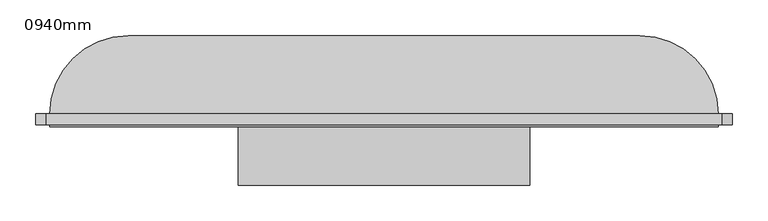
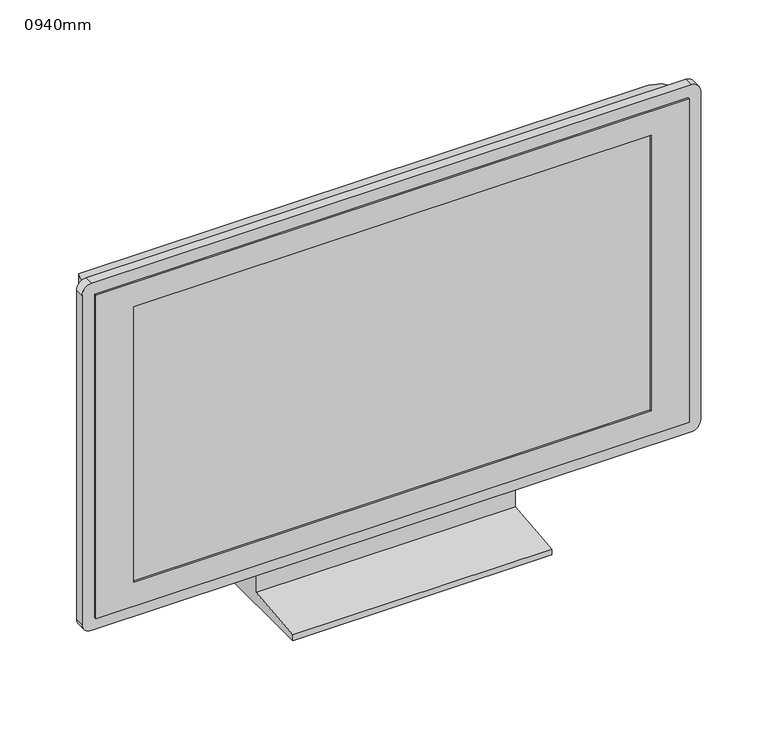
"""IFC4 building model written with IfcOpenShell, lengths in millimetres: furniture geometry, 0940mm."""

from ifc_helpers import new_model, si_unit, point, frame, frame_2d, origin, place, context, project, spatial, polyline, circle_curve, ellipse_curve, trimmed, segment, composite_curve, outline, extrude, faceted_brep, source, transform, mapped, element, save
from ifc_brep_helpers import plane_surface, cylinder_surface, advanced_brep


def furniture_0940mm_4831bac8(model_context):
    return source(origin(), model_context, "Body", "SolidModel", [
        extrude(outline(polyline([(-51.4613764, 80.0), (-1.4613764, 80.0), (48.5386236, 0.0), (-151.4613764, 0.0), (-151.4613764, 10.0), (-51.4613764, 20.0), (-51.4613764, 80.0)])), frame((-208.760248, 0.0, 0.0), z_axis=(1.0, 0.0, 0.0), x_axis=(0.0, 1.0, 0.0)), (0.0, 0.0, 1.0), 409.6314677),
        faceted_brep([(465.6869536, -69.4613764, 620.8776873), (-473.5759818, -69.4613764, 620.8776873), (-473.5759818, -69.4613764, 80.0), (465.6869536, -69.4613764, 80.0), (-413.5759818, -69.4613764, 580.8776873), (405.6869536, -69.4613764, 580.8776873), (405.6869536, -69.4613764, 120.0), (-413.5759818, -69.4613764, 120.0), (465.6869536, -51.4613764, 620.8776873), (465.6869536, -51.4613764, 80.0), (-473.5759818, -51.4613764, 80.0), (-473.5759818, -51.4613764, 620.8776873), (-413.5759818, -66.4613764, 580.8776873), (-413.5759818, -66.4613764, 120.0), (405.6869536, -66.4613764, 120.0), (405.6869536, -66.4613764, 580.8776873)], [[[0, 1, 2, 3], [4, 5, 6, 7]], [[8, 9, 10, 11]], [[1, 0, 8, 11]], [[2, 1, 11, 10]], [[3, 2, 10, 9]], [[0, 3, 9, 8]], [[12, 13, 14, 15]], [[12, 15, 5, 4]], [[15, 14, 6, 5]], [[14, 13, 7, 6]], [[13, 12, 4, 7]]]),
        extrude(outline(composite_curve([segment(polyline([(640.8776873, 470.6869536), (640.8776873, -478.5759818)]), True, "CONTINUOUS"), segment(trimmed(circle_curve(frame_2d((625.8776873, -478.5759818)), 15.0), [point((640.8776873, -478.5759818))], [point((625.8776873, -493.5759818))], False, "CARTESIAN"), True, "CONTINUOUS"), segment(polyline([(625.8776873, -493.5759818), (75.0, -493.5759818)]), True, "CONTINUOUS"), segment(trimmed(circle_curve(frame_2d((75.0, -478.5759818)), 15.0), [point((75.0, -493.5759818))], [point((60.0, -478.5759818))], False, "CARTESIAN"), True, "CONTINUOUS"), segment(polyline([(60.0, -478.5759818), (60.0, 470.6869536)]), True, "CONTINUOUS"), segment(trimmed(circle_curve(frame_2d((75.0, 470.6869536)), 15.0), [point((60.0, 470.6869536))], [point((75.0, 485.6869536))], False, "CARTESIAN"), True, "CONTINUOUS"), segment(polyline([(75.0, 485.6869536), (625.8776873, 485.6869536)]), True, "CONTINUOUS"), segment(trimmed(circle_curve(frame_2d((625.8776873, 470.6869536)), 15.0), [point((625.8776873, 485.6869536))], [point((640.8776873, 470.6869536))], False, "CARTESIAN"), True, "CONTINUOUS")], self_intersect=False), holes=[polyline([(620.8776873, 465.6869536), (80.0, 465.6869536), (80.0, -473.5759818), (620.8776873, -473.5759818), (620.8776873, 465.6869536)])]), frame((0.0, -66.4613764, 0.0), z_axis=(0.0, 1.0, 0.0), x_axis=(0.0, 0.0, 1.0)), (0.0, 0.0, 1.0), 15.0),
        advanced_brep(
        [(-473.5759818, -51.4613764, 80.0), (465.6869536, -51.4613764, 80.0), (465.6869536, -51.4613764, 620.8776873), (-473.5759818, -51.4613764, 620.8776873), (355.6869536, 58.5386236, 80.0), (-363.5759818, 58.5386236, 80.0), (-363.5759818, 58.5386236, 510.8776873), (355.6869536, 58.5386236, 510.8776873)],
        [
            (0, 1),
            (1, 2),
            (2, 3),
            (3, 0),
            (4, 5),
            (5, 6),
            (6, 7),
            (7, 4),
            (0, 5, circle_curve(frame((-363.5759818, -51.4613764, 80.0), z_axis=(0.0, 0.0, -1.0), x_axis=(-1.0, 0.0, 0.0)), 110.0)),
            (4, 1, circle_curve(frame((355.6869536, -51.4613764, 80.0), z_axis=(0.0, 0.0, -1.0), x_axis=(1.0, 0.0, 0.0)), 110.0)),
            (7, 2, ellipse_curve(frame((355.6869536, -51.4613764, 510.8776873), z_axis=(0.7071067811865475, 0.0, -0.7071067811865475), x_axis=(0.7071067811865474, 0.0, 0.7071067811865476)), 155.5634919, 110.0)),
            (6, 3, ellipse_curve(frame((-363.5759818, -51.4613764, 510.8776873), z_axis=(0.7071067811865475, 0.0, 0.7071067811865475), x_axis=(-0.7071067811865476, 0.0, 0.7071067811865474)), 155.5634919, 110.0)),
        ],
        [
            plane_surface(frame((-473.5759818, -51.4613764, 620.8776873), z_axis=(0.0, -1.0, 0.0), x_axis=(-1.0, 0.0, 0.0))),
            plane_surface(frame((-473.5759818, 58.5386236, 620.8776873), z_axis=(0.0, 1.0, 0.0), x_axis=(1.0, 0.0, 0.0))),
            plane_surface(frame((-473.5759818, -51.4613764, 80.0), z_axis=(0.0, 0.0, -1.0), x_axis=(0.0, 1.0, 0.0))),
            cylinder_surface(frame((355.6869536, -51.4613764, 80.0), z_axis=(0.0, 0.0, 1.0), x_axis=(1.0, 0.0, 0.0)), 110.0),
            cylinder_surface(frame((465.6869536, -51.4613764, 510.8776873), z_axis=(-1.0, 0.0, 0.0), x_axis=(0.0, 0.0, 1.0)), 110.0),
            cylinder_surface(frame((-363.5759818, -51.4613764, 620.8776873), z_axis=(0.0, 0.0, -1.0), x_axis=(-1.0, 0.0, 0.0)), 110.0),
        ],
        [
            (0, [[1, 2, 3, 4]]),
            (1, [[5, 6, 7, 8]]),
            (2, [[-1, 9, -5, 10]]),
            (3, [[11, -2, -10, -8]]),
            (4, [[-11, -7, 12, -3]]),
            (5, [[-12, -6, -9, -4]]),
        ],
    ),
    ])


if __name__ == "__main__":
    model = new_model("IFC4")
    model_context = context("Model", 3, world=origin())
    ifc_project = project(units=[si_unit("LENGTHUNIT", "METRE", prefix="MILLI")], contexts=[model_context])
    site = spatial("IfcSite", under=ifc_project)
    building = spatial("IfcBuilding", under=site)
    placement = place(None, origin())
    furniture_0940mm_shape = furniture_0940mm_4831bac8(model_context)
    element("IfcFurniture", 1, ObjectType="0940mm", at=placement, inside=building, context=model_context, shape_type="MappedRepresentation", body=[
        mapped(furniture_0940mm_shape, transform((0.0, 0.0, 0.0), x_axis=(1.0, 0.0, 0.0), y_axis=(0.0, 1.0, 0.0), z_axis=(0.0, 0.0, 1.0))),
    ])
    save(model, "model.ifc")

# Revit data of these elements
# Type "0940mm"
#   SinAng = 0.49 mm
#   L = 819.263 mm
#   H = 460.878 mm
#   Thickness = 110 mm
#   Diagonal = 940 mm
#   CosAng = 0.872 mm
#   Stand [instance default] = yes
#   Default Elevation = 0
# Element 1 (IfcFurniture, "0940mm")
#   Materials on its faces: "TV - Black", "TV - Glass", "TV - Screen"
# Materials
#   "TV - Black": colour RGB 49 49 49, transparency 0
#   "TV - Glass": colour RGB 157 157 157, transparency 0.9
#   "TV - Screen": colour RGB 0 0 0, transparency 0
